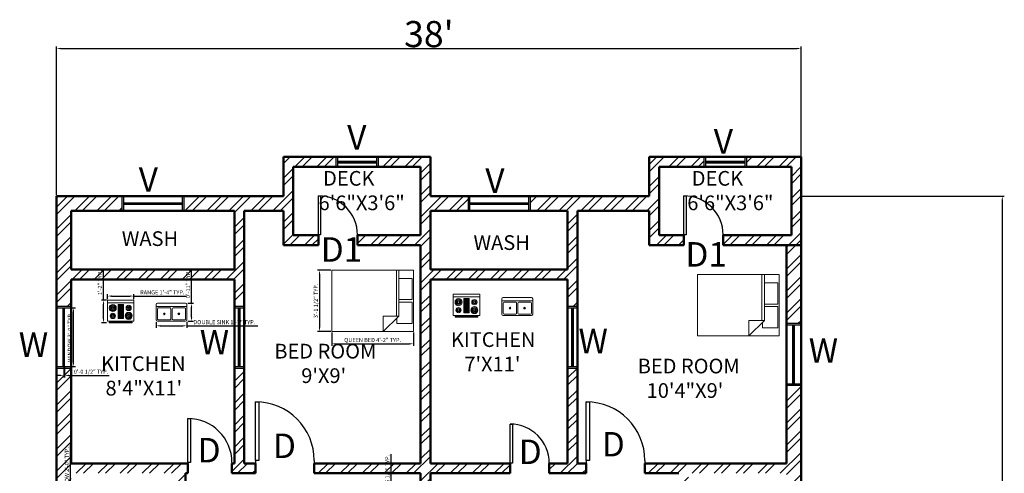
# Model space of a CAD drawing. Units: inches. Extents: x -31438 to -28352, y 12489 to 13610.
# Tile 3 of 5: x -31437 to -30834, y 13238 to 13516. Entities that reach past the tile are written whole.
import ezdxf

# ---------------------------------------------------------------- set-up
doc = ezdxf.new("R2010")
doc.units = ezdxf.units.IN
for name, color, linetype, lineweight in [('A-ANNO-DIMS', 2, 'Continuous', 18), ('A-ANNO-TEXT', 7, 'Continuous', 18), ('A-AREA-IDEN', 3, 'Continuous', 18), ('A-DOOR', 3, 'Continuous', 25), ('A-FLOR-FIXT', 9, 'Continuous', 18), ('A-FURN', 8, 'Continuous', 18), ('A-GLAZ', 4, 'Continuous', 25), ('A-WALL', 7, 'Continuous', 50), ('A-WALL-PATT', 8, 'Continuous', 13)]:
    doc.layers.add(name, color=color, linetype=linetype, lineweight=lineweight)
doc.styles.get("Standard").update_dxf_attribs({"font": 'arial.ttf'})
doc.dimstyles.new('ISO-25', dxfattribs={"dimtxt": 2.5, "dimasz": 2.5, "dimexe": 1.25, "dimexo": 0.625, "dimtad": 1, "dimdec": 0, "dimlunit": 3, "dimtxsty": 'Standard', "dimcen": 2.5, "dimadec": 0, "dimazin": 0, "dimtfac": 1, "dimtdec": 0, "dimtmove": 0, "dimatfit": 3, "dimfxl": 1, "dimarcsym": 0})

# ---------------------------------------------------------------- blocks, each defined once
blk = doc.blocks.new('*U8')
for p, q in [((0, 0), (0, -100)), ((750, 0), (750, -100))]:
    blk.add_line(p, q)
blk.add_lwpolyline([(0, 0), (0, 750), (43.75, 750), (43.75, 0)], close=True)
blk.add_arc((0, 0), 750, 0, 90)
blk = doc.blocks.new('Bed - Queen')
for p, q in [((0, -80.00003), (0, 0)), ((0, 0), (59.99999, 0)), ((59.99999, 0), (59.99999, -80.00003)), ((7.99999, -1.2), (28.79998, -1.2)), ((7.99999, -14.4), (7.99999, -1.2)), ((28.79998, -1.2), (28.79998, -14.4)), ((31.19999, -1.2), (51.99999, -1.2)), ((31.19999, -14.4), (31.19999, -1.2)), ((51.99999, -1.2), (51.99999, -16.4)), ((0, -14.4), (44.8, -14.4)), ((44.8, -16.8), (0, -16.8)), ((59.99999, -29.6), (44.8, -14.4)), ((44.8, -14.4), (44.8, -29.6)), ((51.99999, -16.4), (46.79936, -16.4)), ((44.8, -29.6), (59.99999, -29.6)), ((59.99999, -80.00003), (0, -80.00003))]:
    blk.add_line(p, q)
blk = doc.blocks.new('Range-Oven - 30 in top')
for p, q in [((0, -3), (30, -3)), ((12, -6), (18, -6)), ((13, -20), (13, -6)), ((14, -6), (14, -20)), ((15, -20), (15, -6)), ((16, -6), (16, -20)), ((17, -20), (17, -6)), ((18, -20), (12, -20)), ((6, -24), (6, -25)), ((8, -25), (8, -24)), ((22, -25), (22, -24)), ((24, -24), (24, -25))]:
    blk.add_line(p, q)
for points in [[(0, -24), (0, 0), (30, 0), (30, -24)], [(12, -21), (12, -5), (18, -5), (18, -21)], [(2, -26), (2, -25), (28, -25), (28, -26)]]:
    blk.add_lwpolyline(points, close=True)
for centre, radius in [((6, -9), 4), ((6, -9), 3), ((6, -9), 2), ((6, -9), 1), ((24, -9), 3), ((24, -9), 2), ((24, -9), 1), ((6, -18), 3), ((6, -18), 2), ((6, -18), 1), ((24, -18), 4), ((24, -18), 3), ((24, -18), 2), ((24, -18), 1)]:
    blk.add_circle(centre, radius)
blk = doc.blocks.new('Sink-double - 36 in top')
for p, q in [((-18, -4), (18, -4)), ((-0.75, -18.5), (-0.75, -6.5)), ((0.75, -6.5), (0.75, -18.5))]:
    blk.add_line(p, q)
for points in [[(-16.5, 0), (16.5, 0)], [(-18, -19.5), (-18, -1.5)], [(-16.5, -18.5), (-16.5, -6.5)], [(-15.5, -5.5), (-1.75, -5.5)], [(1.75, -5.5), (15.5, -5.5)], [(16.5, -6.5), (16.5, -18.5)], [(18, -1.5), (18, -19.5)], [(16.5, -21), (-16.5, -21)], [(-1.75, -19.5), (-15.5, -19.5)], [(15.5, -19.5), (1.75, -19.5)]]:
    blk.add_lwpolyline(points)
for centre, radius in [((-8.5, -12.5), 1), ((8.5, -12.5), 1), ((-8.5, -12.5), 0.5), ((8.5, -12.5), 0.5)]:
    blk.add_circle(centre, radius)
for centre, radius, start, end in [((-16.5, -1.5), 1.5, 90, 180), ((16.5, -1.5), 1.5, 0, 90), ((-15.5, -6.5), 1, 90, 180), ((-1.75, -6.5), 1, 0, 90), ((1.75, -6.5), 1, 90, 180), ((15.5, -6.5), 1, 0, 90), ((-16.5, -19.5), 1.5, 180, 270), ((-15.5, -18.5), 1, 180, 270), ((-1.75, -18.5), 1, 270, 0), ((1.75, -18.5), 1, 180, 270), ((15.5, -18.5), 1, 270, 0), ((16.5, -19.5), 1.5, 270, 0)]:
    blk.add_arc(centre, radius, start, end)
blk = doc.blocks.new('*D170')
at = {"layer": 'A-ANNO-DIMS', "color": 0, "lineweight": -2, "transparency": 16777216}
for p, q in [((-31414.86, 13408.54), (-31414.86, 13499.66)), ((-30958.86, 13408.54), (-30958.86, 13499.66)), ((-31412.36, 13498.41), (-30961.36, 13498.41))]:
    blk.add_line(p, q, dxfattribs=at)
at = {"layer": 'A-ANNO-DIMS', "color": 0, "transparency": 16777216}
for points in [[(-31412.36, 13498.83), (-31412.36, 13497.99), (-31414.86, 13498.41)], [(-30961.36, 13498.83), (-30961.36, 13497.99), (-30958.86, 13498.41)]]:
    blk.add_solid(points, dxfattribs=at)
at = {"layer": 'Defpoints', "color": 0, "transparency": 16777216}
for p in [(-30958.86, 13498.41), (-31414.86, 13407.92), (-30958.86, 13407.92)]:
    blk.add_point(p, dxfattribs=at)
at = {"layer": 'A-ANNO-DIMS', "color": 0, "transparency": 16777216, "insert": (-31186.86, 13507.21), "char_height": 2.5, "attachment_point": 5}
blk.add_mtext("{\\H6.4x;38'}", dxfattribs=at)
blk = doc.blocks.new('*D171')
at = {"layer": 'A-ANNO-DIMS', "color": 0, "lineweight": -2, "transparency": 16777216}
for p, q in [((-30958.23, 13407.92), (-30834.47, 13407.92)), ((-30835.72, 13405.42), (-30835.72, 12570.42)), ((-30958.23, 12567.92), (-30834.47, 12567.92))]:
    blk.add_line(p, q, dxfattribs=at)
at = {"layer": 'A-ANNO-DIMS', "color": 0, "transparency": 16777216}
for points in [[(-30836.13, 13405.42), (-30835.3, 13405.42), (-30835.72, 13407.92)], [(-30836.13, 12570.42), (-30835.3, 12570.42), (-30835.72, 12567.92)]]:
    blk.add_solid(points, dxfattribs=at)
at = {"layer": 'Defpoints', "color": 0, "transparency": 16777216}
for p in [(-30958.86, 13407.92), (-30958.86, 12567.92), (-30835.72, 12567.92)]:
    blk.add_point(p, dxfattribs=at)
at = {"layer": 'A-ANNO-DIMS', "color": 0, "transparency": 16777216, "insert": (-30844.51, 12987.92), "char_height": 2.5, "attachment_point": 5, "rotation": 90}
blk.add_mtext("{\\H6.4x;70'}", dxfattribs=at)
blk = doc.blocks.new('WIN-36')
for p, q in [((0, 0), (0, 36)), ((0.5, 0), (0.5, 36))]:
    blk.add_line(p, q)
blk = doc.blocks.new('*D182')
at = {"layer": 'A-ANNO-DIMS', "color": 0, "lineweight": -2, "transparency": 16777216}
for p, q in [((-31209.96, 13225.29), (-31209.96, 13249.87)), ((-31213.84, 13225.29), (-31208.71, 13225.29)), ((-31209.96, 13209.45), (-31209.96, 13222.79)), ((-31213.84, 13206.95), (-31208.71, 13206.95))]:
    blk.add_line(p, q, dxfattribs=at)
at = {"layer": 'A-ANNO-DIMS', "color": 0, "transparency": 16777216}
for points in [[(-31210.38, 13222.79), (-31209.55, 13222.79), (-31209.96, 13225.29)], [(-31210.38, 13209.45), (-31209.55, 13209.45), (-31209.96, 13206.95)]]:
    blk.add_solid(points, dxfattribs=at)
at = {"layer": 'Defpoints', "color": 0, "transparency": 16777216}
for p in [(-31214.46, 13225.29), (-31209.96, 13225.29), (-31214.46, 13206.95)]:
    blk.add_point(p, dxfattribs=at)
at = {"layer": 'A-ANNO-DIMS', "color": 0, "transparency": 16777216, "insert": (-31211.88, 13238.83), "char_height": 2.5, "attachment_point": 5, "rotation": 90}
blk.add_mtext('1\'-6 1/2" TYP.', dxfattribs=at)
blk = doc.blocks.new('*D185')
at = {"layer": 'A-ANNO-DIMS', "color": 0, "lineweight": -2, "transparency": 16777216}
for p, q in [((-31246.31, 13324.33), (-31246.31, 13316.19)), ((-31196.21, 13324.33), (-31196.21, 13316.19)), ((-31243.81, 13317.44), (-31198.71, 13317.44))]:
    blk.add_line(p, q, dxfattribs=at)
at = {"layer": 'A-ANNO-DIMS', "color": 0, "transparency": 16777216}
for points in [[(-31243.81, 13317.86), (-31243.81, 13317.02), (-31246.31, 13317.44)], [(-31198.71, 13317.86), (-31198.71, 13317.02), (-31196.21, 13317.44)]]:
    blk.add_solid(points, dxfattribs=at)
at = {"layer": 'Defpoints', "color": 0, "transparency": 16777216}
for p in [(-31246.31, 13324.96), (-31196.21, 13324.96), (-31196.21, 13317.44)]:
    blk.add_point(p, dxfattribs=at)
at = {"layer": 'A-ANNO-DIMS', "color": 0, "transparency": 16777216, "insert": (-31221.26, 13319.44), "char_height": 2.5, "attachment_point": 5}
blk.add_mtext('QUEEN BED 4\'-2" TYP.', dxfattribs=at)
blk = doc.blocks.new('*D186')
at = {"layer": 'A-ANNO-DIMS', "color": 0, "lineweight": -2, "transparency": 16777216}
for p, q in [((-31246.93, 13362.53), (-31255.07, 13362.53)), ((-31253.82, 13360.03), (-31253.82, 13327.46)), ((-31246.93, 13324.96), (-31255.07, 13324.96))]:
    blk.add_line(p, q, dxfattribs=at)
at = {"layer": 'A-ANNO-DIMS', "color": 0, "transparency": 16777216}
for points in [[(-31254.24, 13360.03), (-31253.41, 13360.03), (-31253.82, 13362.53)], [(-31254.24, 13327.46), (-31253.41, 13327.46), (-31253.82, 13324.96)]]:
    blk.add_solid(points, dxfattribs=at)
at = {"layer": 'Defpoints', "color": 0, "transparency": 16777216}
for p in [(-31246.31, 13362.53), (-31253.82, 13324.96), (-31246.31, 13324.96)]:
    blk.add_point(p, dxfattribs=at)
at = {"layer": 'A-ANNO-DIMS', "color": 0, "transparency": 16777216, "insert": (-31255.74, 13343.74), "char_height": 2.5, "attachment_point": 5, "rotation": 90}
blk.add_mtext('3\'-1 1/2" TYP.', dxfattribs=at)
blk = doc.blocks.new('*D193')
at = {"layer": 'A-ANNO-DIMS', "color": 0, "lineweight": -2, "transparency": 16777216}
for p, q in [((-31406.26, 13220.1), (-31406.26, 13255.48)), ((-31409.23, 13220.1), (-31405.01, 13220.1)), ((-31406.26, 13198.6), (-31406.26, 13217.6)), ((-31409.23, 13196.1), (-31405.01, 13196.1))]:
    blk.add_line(p, q, dxfattribs=at)
at = {"layer": 'A-ANNO-DIMS', "color": 0, "transparency": 16777216}
for points in [[(-31406.67, 13217.6), (-31405.84, 13217.6), (-31406.26, 13220.1)], [(-31406.67, 13198.6), (-31405.84, 13198.6), (-31406.26, 13196.1)]]:
    blk.add_solid(points, dxfattribs=at)
at = {"layer": 'Defpoints', "color": 0, "transparency": 16777216}
for p in [(-31409.86, 13220.1), (-31406.26, 13220.1), (-31409.86, 13196.1)]:
    blk.add_point(p, dxfattribs=at)
at = {"layer": 'A-ANNO-DIMS', "color": 0, "transparency": 16777216, "insert": (-31408.17, 13239.04), "char_height": 2.5, "attachment_point": 5, "rotation": 90}
blk.add_mtext('WINDOW 2\'-0" TYP.', dxfattribs=at)
blk = doc.blocks.new('*D195')
at = {"layer": 'A-ANNO-DIMS', "color": 0, "lineweight": -2, "transparency": 16777216}
for p, q in [((-31409.23, 13339.51), (-31403.21, 13339.51)), ((-31404.46, 13306.01), (-31404.46, 13337.01)), ((-31409.23, 13303.51), (-31403.21, 13303.51))]:
    blk.add_line(p, q, dxfattribs=at)
at = {"layer": 'A-ANNO-DIMS', "color": 0, "transparency": 16777216}
for points in [[(-31404.87, 13337.01), (-31404.04, 13337.01), (-31404.46, 13339.51)], [(-31404.87, 13306.01), (-31404.04, 13306.01), (-31404.46, 13303.51)]]:
    blk.add_solid(points, dxfattribs=at)
at = {"layer": 'Defpoints', "color": 0, "transparency": 16777216}
for p in [(-31409.86, 13339.51), (-31404.46, 13339.51), (-31409.86, 13303.51)]:
    blk.add_point(p, dxfattribs=at)
at = {"layer": 'A-ANNO-DIMS', "color": 0, "transparency": 16777216, "insert": (-31406.38, 13321.51), "char_height": 2.5, "attachment_point": 5, "rotation": 90}
blk.add_mtext('WINDOW 3\'-0" TYP.', dxfattribs=at)
blk = doc.blocks.new('*D196')
at = {"layer": 'A-ANNO-DIMS', "color": 0, "lineweight": -2, "transparency": 16777216}
for p, q in [((-31410.36, 13302.88), (-31410.36, 13296.86)), ((-31409.86, 13302.88), (-31409.86, 13296.86)), ((-31412.86, 13298.11), (-31415.36, 13298.11)), ((-31410.36, 13298.11), (-31409.86, 13298.11)), ((-31407.36, 13298.11), (-31382.54, 13298.11))]:
    blk.add_line(p, q, dxfattribs=at)
at = {"layer": 'A-ANNO-DIMS', "color": 0, "transparency": 16777216}
for points in [[(-31412.86, 13298.52), (-31412.86, 13297.69), (-31410.36, 13298.11)], [(-31407.36, 13298.52), (-31407.36, 13297.69), (-31409.86, 13298.11)]]:
    blk.add_solid(points, dxfattribs=at)
at = {"layer": 'Defpoints', "color": 0, "transparency": 16777216}
for p in [(-31410.36, 13303.51), (-31409.86, 13303.51), (-31409.86, 13298.11)]:
    blk.add_point(p, dxfattribs=at)
at = {"layer": 'A-ANNO-DIMS', "color": 0, "transparency": 16777216, "insert": (-31393.7, 13300.02), "char_height": 2.5, "attachment_point": 5}
blk.add_mtext('0\'-0 1/2" TYP.', dxfattribs=at)
blk = doc.blocks.new('*D197')
at = {"layer": 'A-ANNO-DIMS', "color": 0, "lineweight": -2, "transparency": 16777216}
for p, q in [((-31383.61, 13344.88), (-31383.61, 13347.94)), ((-31381.11, 13346.69), (-31369.92, 13346.69)), ((-31367.42, 13344.88), (-31367.42, 13347.94)), ((-31367.42, 13346.69), (-31335.17, 13346.69))]:
    blk.add_line(p, q, dxfattribs=at)
at = {"layer": 'A-ANNO-DIMS', "color": 0, "transparency": 16777216}
for points in [[(-31381.11, 13347.11), (-31381.11, 13346.27), (-31383.61, 13346.69)], [(-31369.92, 13347.11), (-31369.92, 13346.27), (-31367.42, 13346.69)]]:
    blk.add_solid(points, dxfattribs=at)
at = {"layer": 'Defpoints', "color": 0, "transparency": 16777216}
for p in [(-31383.61, 13344.26), (-31367.42, 13346.69), (-31367.42, 13344.26)]:
    blk.add_point(p, dxfattribs=at)
at = {"layer": 'A-ANNO-DIMS', "color": 0, "transparency": 16777216, "insert": (-31350.04, 13348.61), "char_height": 2.5, "attachment_point": 5}
blk.add_mtext('RANGE 1\'-4" TYP.', dxfattribs=at)
blk = doc.blocks.new('*D198')
at = {"layer": 'A-ANNO-DIMS', "color": 0, "lineweight": -2, "transparency": 16777216}
for p, q in [((-31386.04, 13344.26), (-31386.04, 13363.01)), ((-31384.24, 13344.26), (-31387.29, 13344.26)), ((-31386.04, 13332.72), (-31386.04, 13341.76)), ((-31384.24, 13330.22), (-31387.29, 13330.22))]:
    blk.add_line(p, q, dxfattribs=at)
at = {"layer": 'A-ANNO-DIMS', "color": 0, "transparency": 16777216}
for points in [[(-31386.46, 13341.76), (-31385.62, 13341.76), (-31386.04, 13344.26)], [(-31386.46, 13332.72), (-31385.62, 13332.72), (-31386.04, 13330.22)]]:
    blk.add_solid(points, dxfattribs=at)
at = {"layer": 'Defpoints', "color": 0, "transparency": 16777216}
for p in [(-31386.04, 13344.26), (-31383.61, 13344.26), (-31383.61, 13330.22)]:
    blk.add_point(p, dxfattribs=at)
at = {"layer": 'A-ANNO-DIMS', "color": 0, "transparency": 16777216, "insert": (-31387.92, 13354.89), "char_height": 2.5, "attachment_point": 5, "rotation": 90}
blk.add_mtext('1\'-2" TYP.', dxfattribs=at)
blk = doc.blocks.new('*D205')
at = {"layer": 'A-ANNO-DIMS', "color": 0, "lineweight": -2, "transparency": 16777216}
for p, q in [((-31353.83, 13330.68), (-31353.83, 13327.23)), ((-31334.97, 13330.68), (-31334.97, 13327.23)), ((-31351.33, 13328.48), (-31337.47, 13328.48)), ((-31334.97, 13328.48), (-31291.66, 13328.48))]:
    blk.add_line(p, q, dxfattribs=at)
at = {"layer": 'A-ANNO-DIMS', "color": 0, "transparency": 16777216}
for points in [[(-31351.33, 13328.89), (-31351.33, 13328.06), (-31353.83, 13328.48)], [(-31337.47, 13328.89), (-31337.47, 13328.06), (-31334.97, 13328.48)]]:
    blk.add_solid(points, dxfattribs=at)
at = {"layer": 'Defpoints', "color": 0, "transparency": 16777216}
for p in [(-31353.83, 13331.3), (-31334.97, 13331.3), (-31334.97, 13328.48)]:
    blk.add_point(p, dxfattribs=at)
at = {"layer": 'A-ANNO-DIMS', "color": 0, "transparency": 16777216, "insert": (-31312.07, 13330.39), "char_height": 2.5, "attachment_point": 5}
blk.add_mtext('DOUBLE SINK 1\'-7" TYP.', dxfattribs=at)
blk = doc.blocks.new('*D206')
at = {"layer": 'A-ANNO-DIMS', "color": 0, "lineweight": -2, "transparency": 16777216}
for p, q in [((-31332.15, 13342.3), (-31332.15, 13363.23)), ((-31334.35, 13342.3), (-31330.9, 13342.3)), ((-31332.15, 13333.8), (-31332.15, 13339.8)), ((-31334.35, 13331.3), (-31330.9, 13331.3))]:
    blk.add_line(p, q, dxfattribs=at)
at = {"layer": 'A-ANNO-DIMS', "color": 0, "transparency": 16777216}
for points in [[(-31332.56, 13339.8), (-31331.73, 13339.8), (-31332.15, 13342.3)], [(-31332.56, 13333.8), (-31331.73, 13333.8), (-31332.15, 13331.3)]]:
    blk.add_solid(points, dxfattribs=at)
at = {"layer": 'Defpoints', "color": 0, "transparency": 16777216}
for p in [(-31334.97, 13342.3), (-31332.15, 13342.3), (-31334.97, 13331.3)]:
    blk.add_point(p, dxfattribs=at)
at = {"layer": 'A-ANNO-DIMS', "color": 0, "transparency": 16777216, "insert": (-31334.05, 13354.02), "char_height": 2.5, "attachment_point": 5, "rotation": 90}
blk.add_mtext('0\'-11" TYP.', dxfattribs=at)

msp = doc.modelspace()

# ---------------------------------------------------------------- hatches: boundary and pattern name
at = {"layer": 'A-WALL-PATT'}
h = msp.add_hatch(dxfattribs=at)
h.set_pattern_fill('ANSI32', color=256)
h.paths.add_polyline_path([(-30958.86, 13431.92), (-30992.36, 13431.92), (-30992.36, 13425.92), (-30964.86, 13425.92), (-30964.86, 13383.92), (-31006.63, 13383.92), (-31006.63, 13380.92), (-31006.63, 13377.92), (-30958.86, 13377.92)])
h.paths.add_polyline_path([(-30958.86, 13377.92), (-30967.86, 13377.92), (-30967.86, 13330.01), (-30958.86, 13330.01)])
h.paths.add_polyline_path([(-31018.36, 13431.92), (-31051.86, 13431.92), (-31051.86, 13407.92), (-31124.86, 13407.92), (-31124.86, 13398.92), (-31101.86, 13398.92), (-31101.86, 13362.92), (-31185.86, 13362.92), (-31185.86, 13398.92), (-31162.86, 13398.92), (-31162.86, 13407.92), (-31185.86, 13407.92), (-31185.86, 13431.92), (-31217.86, 13431.92), (-31217.86, 13425.92), (-31191.86, 13425.92), (-31191.86, 13383.92), (-31230.51, 13383.92), (-31230.51, 13377.92), (-31191.86, 13377.92), (-31191.86, 13244.1), (-31256.99, 13244.1), (-31256.99, 13238.1), (-31191.86, 13238.1), (-31191.86, 13183.6), (-31185.86, 13183.6), (-31185.86, 13238.1), (-31137.12, 13238.1), (-31137.12, 13244.1), (-31185.86, 13244.1), (-31185.86, 13356.92), (-31101.86, 13356.92), (-31101.86, 13340.51), (-31095.86, 13340.51), (-31095.86, 13398.92), (-31051.86, 13398.92), (-31051.86, 13377.92), (-31030.63, 13377.92), (-31030.63, 13383.92), (-31045.86, 13383.92), (-31045.86, 13425.92), (-31018.36, 13425.92)])
h.paths.add_polyline_path([(-31269.86, 13425.92), (-31243.86, 13425.92), (-31243.86, 13431.92), (-31275.86, 13431.92), (-31275.86, 13407.92), (-31336.86, 13407.92), (-31336.86, 13398.92), (-31305.86, 13398.92), (-31305.86, 13362.92), (-31405.86, 13362.92), (-31405.86, 13398.92), (-31374.86, 13398.92), (-31374.86, 13407.92), (-31414.86, 13407.92), (-31414.86, 13340.51), (-31405.86, 13340.51), (-31405.86, 13356.92), (-31305.86, 13356.92), (-31305.86, 13340.51), (-31299.86, 13340.51), (-31299.86, 13398.92), (-31275.86, 13398.92), (-31275.86, 13377.92), (-31254.51, 13377.92), (-31254.51, 13383.92), (-31269.86, 13383.92)])
h.paths.add_polyline_path([(-31299.86, 13302.51), (-31305.86, 13302.51), (-31305.86, 13244.1), (-31307.44, 13244.1), (-31307.44, 13241.1), (-31307.44, 13238.1), (-31292.99, 13238.1), (-31292.99, 13244.1), (-31299.86, 13244.1)])
h.paths.add_polyline_path([(-31334.44, 13244.1), (-31405.86, 13244.1), (-31405.86, 13302.51), (-31414.86, 13302.51), (-31414.86, 13221.1), (-31405.86, 13221.1), (-31405.86, 13238.1), (-31341.86, 13238.1), (-31341.86, 13213.77), (-31335.86, 13213.77), (-31335.86, 13238.1), (-31334.44, 13238.1)])
h.paths.add_polyline_path([(-31090.53, 13244.1), (-31095.86, 13244.1), (-31095.86, 13302.51), (-31101.86, 13302.51), (-31101.86, 13244.1), (-31113.12, 13244.1), (-31113.12, 13241.1), (-31113.12, 13238.1), (-31090.53, 13238.1)], flags=17)
h.paths.add_polyline_path([(-30958.86, 13292.01), (-30967.86, 13292.01), (-30967.86, 13244.1), (-31033.86, 13244.1), (-31054.53, 13244.1), (-31054.53, 13241.1), (-31054.53, 13238.1), (-31033.86, 13238.1), (-31033.86, 13218.45), (-31027.86, 13218.45), (-31027.86, 13238.1), (-30967.86, 13238.1), (-30967.86, 13221.1), (-30958.86, 13221.1)])
h.paths.add_polyline_path([(-30958.86, 13195.1), (-30967.86, 13195.1), (-30967.86, 13178.1), (-31027.86, 13178.1), (-31027.86, 13194.45), (-31030.86, 13194.45), (-31033.86, 13194.45), (-31033.86, 13162.82), (-31027.86, 13162.82), (-31027.86, 13172.1), (-30967.86, 13172.1), (-30967.86, 13147.51), (-30958.86, 13147.51)])
h.paths.add_polyline_path([(-30958.86, 13121.51), (-30967.86, 13121.51), (-30967.86, 13096.92), (-31027.86, 13096.92), (-31027.86, 13128.82), (-31033.86, 13128.82), (-31033.86, 13096.92), (-31037.31, 13096.92), (-31037.31, 13090.92), (-30967.86, 13090.92), (-30967.86, 13067.92), (-30958.86, 13067.92)])
h.paths.add_polyline_path([(-30958.86, 13029.92), (-30967.86, 13029.92), (-30967.86, 13006.92), (-31025.37, 13006.92), (-31095.86, 13006.92), (-31095.86, 13000.92), (-31081.86, 13000.92), (-31081.86, 12943.92), (-31095.86, 12943.92), (-31095.86, 12937.92), (-31081.86, 12937.92), (-31081.86, 12894.3), (-31075.86, 12894.3), (-31075.86, 13000.92), (-31025.37, 13000.92), (-30967.86, 13000.92), (-30967.86, 12946.42), (-30958.86, 12946.42)])
h.paths.add_polyline_path([(-31121.86, 13006.92), (-31135.86, 13006.92), (-31135.86, 13090.92), (-31081.86, 13090.92), (-31081.86, 13068.53), (-31075.86, 13068.53), (-31075.86, 13090.92), (-31073.31, 13090.92), (-31073.31, 13096.92), (-31141.86, 13096.92), (-31141.86, 13091.1), (-31147.29, 13091.1), (-31147.29, 13085.1), (-31141.86, 13085.1), (-31141.86, 12949.88), (-31146.05, 12949.88), (-31146.05, 12943.88), (-31141.86, 12943.88), (-31141.86, 12853.92), (-31185.86, 12853.92), (-31185.86, 12943.88), (-31182.05, 12943.88), (-31182.05, 12949.88), (-31192.89, 12949.88), (-31192.89, 12943.88), (-31191.86, 12943.88), (-31191.86, 12853.92), (-31231.86, 12853.92), (-31231.86, 12943.88), (-31228.89, 12943.88), (-31228.89, 12949.88), (-31231.86, 12949.88), (-31231.86, 12979.92), (-31272.86, 12979.92), (-31272.86, 12973.92), (-31237.86, 12973.92), (-31237.86, 12853.92), (-31298, 12853.92), (-31298, 12847.92), (-31191.86, 12847.92), (-31191.86, 12806.42), (-31185.86, 12806.42), (-31185.86, 12847.92), (-31074.17, 12847.92), (-31074.17, 12853.92), (-31075.86, 12853.92), (-31075.86, 12870.3), (-31081.86, 12870.3), (-31081.86, 12853.92), (-31135.86, 12853.92), (-31135.86, 12937.92), (-31121.86, 12937.92), (-31121.86, 12943.92), (-31135.86, 12943.92), (-31135.86, 13000.92), (-31121.86, 13000.92)])
h.paths.add_polyline_path([(-30958.86, 12908.42), (-30967.86, 12908.42), (-30967.86, 12853.92), (-31038.17, 12853.92), (-31038.17, 12850.92), (-31038.17, 12847.92), (-31033.86, 12847.92), (-31033.86, 12837.06), (-31027.86, 12837.06), (-31027.86, 12847.92), (-30967.86, 12847.92), (-30967.86, 12833.42), (-30958.86, 12833.42)])
h.paths.add_polyline_path([(-30958.86, 12807.42), (-30967.86, 12807.42), (-30967.86, 12792.92), (-31027.86, 12792.92), (-31027.86, 12803.06), (-31033.86, 12803.06), (-31033.86, 12773.49), (-31027.86, 12773.49), (-31027.86, 12786.92), (-30967.86, 12786.92), (-30967.86, 12769.92), (-30958.86, 12769.92)])
h.paths.add_polyline_path([(-30958.86, 12743.92), (-30967.86, 12743.92), (-30967.86, 12726.92), (-31027.86, 12726.92), (-31027.86, 12749.49), (-31033.86, 12749.49), (-31033.86, 12726.92), (-31035.47, 12726.92), (-31035.47, 12720.92), (-30967.86, 12720.92), (-30967.86, 12667.92), (-30958.86, 12667.92)])
h.paths.add_polyline_path([(-30958.86, 12629.92), (-30967.86, 12629.92), (-30967.86, 12618.92), (-31071.86, 12618.92), (-31071.86, 12612.92), (-30967.86, 12612.92), (-30967.86, 12576.92), (-31000.86, 12576.92), (-31000.86, 12567.92), (-30958.86, 12567.92)])
h.paths.add_polyline_path([(-31038.86, 12576.92), (-31071.86, 12576.92), (-31071.86, 12629.92), (-31077.86, 12629.92), (-31077.86, 12576.92), (-31101.86, 12576.92), (-31101.86, 12597.92), (-31115.03, 12597.92), (-31115.03, 12591.92), (-31107.86, 12591.92), (-31107.86, 12549.92), (-31133.86, 12549.92), (-31133.86, 12543.92), (-31101.86, 12543.92), (-31101.86, 12567.92), (-31038.86, 12567.92)])
h.paths.add_polyline_path([(-31159.86, 12549.92), (-31185.86, 12549.92), (-31185.86, 12591.92), (-31139.03, 12591.92), (-31139.03, 12597.92), (-31185.86, 12597.92), (-31185.86, 12720.92), (-31126.49, 12720.92), (-31126.49, 12726.92), (-31185.86, 12726.92), (-31185.86, 12768.42), (-31191.86, 12768.42), (-31191.86, 12726.92), (-31226.35, 12726.92), (-31226.35, 12720.92), (-31191.86, 12720.92), (-31191.86, 12618.92), (-31275.86, 12618.92), (-31275.86, 12720.92), (-31262.35, 12720.92), (-31262.35, 12726.92), (-31298.57, 12726.92), (-31298.57, 12720.92), (-31281.86, 12720.92), (-31281.86, 12576.92), (-31321.86, 12576.92), (-31321.86, 12597.92), (-31340.38, 12597.92), (-31340.38, 12591.92), (-31327.86, 12591.92), (-31327.86, 12549.92), (-31355.36, 12549.92), (-31355.36, 12543.92), (-31321.86, 12543.92), (-31321.86, 12567.92), (-31252.86, 12567.92), (-31252.86, 12576.92), (-31275.86, 12576.92), (-31275.86, 12612.92), (-31191.86, 12612.92), (-31191.86, 12576.92), (-31214.86, 12576.92), (-31214.86, 12567.92), (-31191.86, 12567.92), (-31191.86, 12543.92), (-31159.86, 12543.92)])
h.paths.add_polyline_path([(-31071.86, 12720.92), (-31071.47, 12726.92), (-31090.49, 12726.92), (-31090.49, 12720.92), (-31077.86, 12720.92), (-31077.86, 12667.92), (-31071.86, 12667.92)])
h.paths.add_polyline_path([(-31381.36, 12549.92), (-31408.86, 12549.92), (-31408.86, 12591.92), (-31364.38, 12591.92), (-31364.38, 12597.92), (-31414.86, 12597.92), (-31414.86, 12543.92), (-31381.36, 12543.92)])
h.paths.add_polyline_path([(-31405.86, 12640.42), (-31414.86, 12640.42), (-31414.86, 12597.92), (-31405.86, 12597.92)])
h.paths.add_polyline_path([(-31405.86, 12720.92), (-31334.57, 12720.92), (-31334.57, 12726.92), (-31339.86, 12726.92), (-31339.86, 12750.16), (-31345.86, 12750.16), (-31345.86, 12726.92), (-31405.86, 12726.92), (-31405.86, 12743.92), (-31414.86, 12743.92), (-31414.86, 12678.42), (-31405.86, 12678.42)])
h.paths.add_polyline_path([(-31339.86, 12806.09), (-31345.86, 12806.09), (-31345.86, 12792.92), (-31405.86, 12792.92), (-31405.86, 12807.42), (-31414.86, 12807.42), (-31414.86, 12769.92), (-31405.86, 12769.92), (-31405.86, 12786.92), (-31345.86, 12786.92), (-31345.86, 12774.16), (-31339.86, 12774.16)])
h.paths.add_polyline_path([(-31334, 12853.92), (-31345.86, 12853.92), (-31345.86, 12973.92), (-31310.86, 12973.92), (-31310.86, 12979.92), (-31405.86, 12979.92), (-31405.86, 13013.51), (-31414.86, 13013.51), (-31414.86, 12971.92), (-31405.86, 12971.92), (-31405.86, 12970.92), (-31409.86, 12970.92), (-31409.86, 12946.92), (-31410.86, 12946.92), (-31410.86, 12970.92), (-31414.86, 12970.92), (-31414.86, 12883.92), (-31405.86, 12883.92), (-31405.86, 12882.92), (-31414.86, 12882.92), (-31414.86, 12833.42), (-31405.86, 12833.42), (-31405.86, 12847.92), (-31345.86, 12847.92), (-31345.86, 12840.09), (-31339.86, 12840.09), (-31339.86, 12847.92), (-31334, 12847.92)])
h.paths.add_polyline_path([(-31351.86, 12937.92), (-31359.89, 12937.92), (-31359.89, 12943.92), (-31351.86, 12943.92), (-31351.86, 12973.92), (-31405.86, 12973.92), (-31405.86, 12943.92), (-31383.89, 12943.92), (-31383.89, 12937.92), (-31405.86, 12937.92), (-31405.86, 12853.92), (-31351.86, 12853.92)], flags=16)
h.paths.add_polyline_path([(-31386.16, 12876.52), (-31390.61, 12876.52), (-31389.24, 12872.41, -0.501323), (-31392.64, 12859.49, -0.132891), (-31394.07, 12859.49, -0.501317), (-31397.46, 12872.41), (-31396.09, 12876.52), (-31398.15, 12876.52), (-31398.15, 12875.49), (-31400.2, 12875.49), (-31400.2, 12876.18), (-31400.22, 12876.52), (-31400.54, 12876.52), (-31400.54, 12882), (-31386.16, 12882)], flags=0)
h.paths.add_polyline_path([(-31387.36, 12877.2), (-31399.17, 12877.2, -0.414214), (-31399.86, 12877.72), (-31399.86, 12880.63, -0.414214), (-31399.35, 12881.31), (-31387.53, 12881.31, -0.414214), (-31386.85, 12880.8), (-31386.85, 12877.89, -0.414214)], flags=0)
h.paths.add_polyline_path([(-31392.23, 12860.41, -0.215004), (-31394.48, 12860.41, -0.48008), (-31396.09, 12872.41), (-31390.61, 12872.41, -0.48008)], flags=0)
h.paths.add_polyline_path([(-31359.87, 12913.86), (-31361.27, 12913.86), (-31361.27, 12937.86), (-31359.87, 12937.86)], flags=0)
h.paths.add_polyline_path([(-31230.55, 13091.1), (-31335.86, 13091.1), (-31335.86, 13129.57), (-31341.86, 13129.57), (-31341.86, 13091.1), (-31405.86, 13091.1), (-31405.86, 13118.6), (-31414.86, 13118.6), (-31414.86, 13051.51), (-31405.86, 13051.51), (-31405.86, 13085.1), (-31230.55, 13085.1)])
h.paths.add_polyline_path([(-31335.86, 13189.77), (-31341.86, 13189.77), (-31341.86, 13178.1), (-31405.86, 13178.1), (-31405.86, 13195.1), (-31414.86, 13195.1), (-31414.86, 13144.6), (-31405.86, 13144.6), (-31405.86, 13172.1), (-31341.86, 13172.1), (-31341.86, 13163.57), (-31335.86, 13163.57)])
h.paths.add_polyline_path([(-31387.11, 12934.37), (-31352.82, 12934.37), (-31352.82, 12965.28), (-31387.11, 12965.28)], flags=8)
h.paths.add_polyline_path([(-31406.38, 12887.22), (-31351.66, 12887.22), (-31351.66, 12920.8), (-31406.38, 12920.8)], flags=24)

# ---------------------------------------------------------------- linework, layer by layer
at = {"layer": 'A-GLAZ'}
for p, q in [((-31243.86, 13431.92), (-31243.86, 13425.92)), ((-31242.86, 13431.92), (-31242.86, 13425.92)), ((-31242.86, 13429.42), (-31218.86, 13429.42)), ((-31242.86, 13428.92), (-31218.86, 13428.92)), ((-31242.86, 13428.42), (-31218.86, 13428.42)), ((-31218.86, 13431.92), (-31218.86, 13425.92)), ((-31217.86, 13431.92), (-31217.86, 13425.92)), ((-31018.36, 13431.92), (-31018.36, 13425.92)), ((-31017.36, 13431.92), (-31017.36, 13425.92)), ((-31017.36, 13429.42), (-30993.36, 13429.42)), ((-31017.36, 13428.92), (-30993.36, 13428.92)), ((-31017.36, 13428.42), (-30993.36, 13428.42)), ((-30993.36, 13431.92), (-30993.36, 13425.92)), ((-30992.36, 13431.92), (-30992.36, 13425.92)), ((-31374.86, 13407.92), (-31374.86, 13398.92)), ((-31373.86, 13407.92), (-31373.86, 13398.92)), ((-31373.86, 13403.92), (-31337.86, 13403.92)), ((-31337.86, 13407.92), (-31337.86, 13398.92)), ((-31336.86, 13407.92), (-31336.86, 13398.92)), ((-31162.86, 13407.92), (-31162.86, 13398.92)), ((-31161.86, 13407.92), (-31161.86, 13398.92)), ((-31161.86, 13403.92), (-31125.86, 13403.92)), ((-31125.86, 13407.92), (-31125.86, 13398.92)), ((-31124.86, 13407.92), (-31124.86, 13398.92)), ((-31414.86, 13340.51), (-31405.86, 13340.51)), ((-31414.86, 13339.51), (-31405.86, 13339.51)), ((-31410.86, 13303.51), (-31410.86, 13339.51)), ((-31305.86, 13340.51), (-31299.86, 13340.51)), ((-31305.86, 13339.51), (-31299.86, 13339.51)), ((-31303.36, 13303.51), (-31303.36, 13339.51)), ((-31302.86, 13303.51), (-31302.86, 13339.51)), ((-31302.36, 13303.51), (-31302.36, 13339.51)), ((-31101.86, 13340.51), (-31095.86, 13340.51)), ((-31101.86, 13339.51), (-31095.86, 13339.51)), ((-31099.36, 13303.51), (-31099.36, 13339.51)), ((-31098.86, 13303.51), (-31098.86, 13339.51)), ((-31098.36, 13303.51), (-31098.36, 13339.51)), ((-30967.86, 13330.01), (-30958.86, 13330.01)), ((-30967.86, 13329.01), (-30958.86, 13329.01)), ((-30963.86, 13293.01), (-30963.86, 13329.01)), ((-31414.86, 13303.51), (-31405.86, 13303.51)), ((-31414.86, 13302.51), (-31405.86, 13302.51)), ((-31305.86, 13303.51), (-31299.86, 13303.51)), ((-31305.86, 13302.51), (-31299.86, 13302.51)), ((-31101.86, 13303.51), (-31095.86, 13303.51)), ((-31101.86, 13302.51), (-31095.86, 13302.51)), ((-30967.86, 13293.01), (-30958.86, 13293.01)), ((-30967.86, 13292.01), (-30958.86, 13292.01))]:
    msp.add_line(p, q, dxfattribs=at)
at = {"layer": 'A-WALL'}
for p, q in [((-31275.86, 13431.92), (-31185.86, 13431.92)), ((-31275.86, 13407.92), (-31275.86, 13431.92)), ((-31185.86, 13407.92), (-31185.86, 13431.92)), ((-31051.86, 13431.92), (-31051.86, 13407.92)), ((-31051.86, 13431.92), (-30958.86, 13431.92)), ((-30958.86, 13431.92), (-30958.86, 12567.92)), ((-31269.86, 13425.92), (-31191.86, 13425.92)), ((-31269.86, 13383.92), (-31269.86, 13425.92)), ((-31191.86, 13383.92), (-31191.86, 13425.92)), ((-31045.86, 13425.92), (-31045.86, 13383.92)), ((-31045.86, 13425.92), (-30964.86, 13425.92)), ((-30964.86, 13425.92), (-30964.86, 13383.92)), ((-31414.86, 13407.92), (-31275.86, 13407.92)), ((-31414.86, 12543.92), (-31414.86, 13407.92)), ((-31185.86, 13407.92), (-31051.86, 13407.92)), ((-31405.86, 13398.92), (-31305.86, 13398.92)), ((-31405.86, 13362.92), (-31405.86, 13398.92)), ((-31305.86, 13362.92), (-31305.86, 13398.92)), ((-31299.86, 13244.1), (-31299.86, 13398.92)), ((-31299.86, 13398.92), (-31275.86, 13398.92)), ((-31275.86, 13377.92), (-31275.86, 13398.92)), ((-31185.86, 13398.92), (-31101.86, 13398.92)), ((-31185.86, 13362.92), (-31185.86, 13398.92)), ((-31101.86, 13362.92), (-31101.86, 13398.92)), ((-31095.86, 13244.1), (-31095.86, 13398.92)), ((-31095.86, 13398.92), (-31051.86, 13398.92)), ((-31051.86, 13398.92), (-31051.86, 13377.92)), ((-31269.86, 13383.92), (-31254.51, 13383.92)), ((-31254.51, 13383.92), (-31254.51, 13377.92)), ((-31230.51, 13383.92), (-31230.51, 13377.92)), ((-31230.51, 13383.92), (-31191.86, 13383.92)), ((-31045.86, 13383.92), (-31030.63, 13383.92)), ((-31030.63, 13383.92), (-31030.63, 13377.92)), ((-31006.63, 13383.92), (-31006.63, 13377.92)), ((-31006.63, 13383.92), (-30964.86, 13383.92)), ((-31275.86, 13377.92), (-31254.51, 13377.92)), ((-31230.51, 13377.92), (-31191.86, 13377.92)), ((-31191.86, 13244.1), (-31191.86, 13377.92)), ((-31051.86, 13377.92), (-31030.63, 13377.92)), ((-31006.63, 13377.92), (-30958.86, 13377.92)), ((-30967.86, 13377.92), (-30967.86, 13244.1)), ((-31405.86, 13362.92), (-31305.86, 13362.92)), ((-31185.86, 13362.92), (-31101.86, 13362.92)), ((-31405.86, 13244.1), (-31405.86, 13356.92)), ((-31405.86, 13356.92), (-31305.86, 13356.92)), ((-31305.86, 13244.1), (-31305.86, 13356.92)), ((-31185.86, 13244.1), (-31185.86, 13356.92)), ((-31185.86, 13356.92), (-31101.86, 13356.92)), ((-31101.86, 13244.1), (-31101.86, 13356.92)), ((-31334.44, 13244.1), (-31405.86, 13244.1)), ((-31334.44, 13244.1), (-31334.44, 13238.1)), ((-31305.86, 13244.1), (-31307.44, 13244.1)), ((-31307.44, 13244.1), (-31307.44, 13238.1)), ((-31292.99, 13244.1), (-31299.86, 13244.1)), ((-31292.99, 13244.1), (-31292.99, 13238.1)), ((-31191.86, 13244.1), (-31256.99, 13244.1)), ((-31256.99, 13244.1), (-31256.99, 13238.1)), ((-31137.12, 13244.1), (-31185.86, 13244.1)), ((-31137.12, 13244.1), (-31137.12, 13238.1)), ((-31101.86, 13244.1), (-31113.12, 13244.1)), ((-31113.12, 13244.1), (-31113.12, 13238.1)), ((-31090.53, 13244.1), (-31095.86, 13244.1)), ((-31090.53, 13244.1), (-31090.53, 13238.1)), ((-31033.86, 13244.1), (-31054.53, 13244.1)), ((-31054.53, 13244.1), (-31054.53, 13238.1)), ((-30967.86, 13244.1), (-31033.86, 13244.1)), ((-31334.44, 13238.1), (-31335.86, 13238.1)), ((-31335.86, 13213.77), (-31335.86, 13238.1)), ((-31292.99, 13238.1), (-31307.44, 13238.1)), ((-31191.86, 13238.1), (-31256.99, 13238.1)), ((-31191.86, 13091.1), (-31191.86, 13238.1)), ((-31185.86, 13091.1), (-31185.86, 13238.1)), ((-31137.12, 13238.1), (-31185.86, 13238.1)), ((-31090.53, 13238.1), (-31113.12, 13238.1)), ((-31033.86, 13238.1), (-31054.53, 13238.1))]:
    msp.add_line(p, q, dxfattribs=at)

# ---------------------------------------------------------------- block references
at = {"layer": 'A-DOOR'}
for p, xscale, yscale, zscale in [((-31254.51, 13384.12), 0.0319999999999912, 0.0319999999999912, 0.0319999999999912), ((-31030.63, 13384.12), 0.0319999999999912, 0.0319999999999912, 0.0319999999999912), ((-31292.99, 13245.9), 0.0480000000000013, 0.0480000000000013, 0.0480000000000013), ((-31090.53, 13245.9), 0.0480000000000013, 0.0480000000000013, 0.0480000000000013), ((-31334.44, 13244.7), 0.036000000000001, 0.036000000000001, 0.036000000000001), ((-31137.12, 13244.3), 0.0319999999999686, 0.0319999999999686, 0.0319999999999686)]:
    msp.add_blockref('*U8', p, dxfattribs=dict(at, xscale=xscale, yscale=yscale, zscale=zscale))
at = {"layer": 'A-FLOR-FIXT'}
for name, p, xscale, yscale, zscale in [('Range-Oven - 30 in top', (-31383.61, 13344.26), 0.5398294676678127, 0.5398294676678127, 0.5398294676678127), ('Range-Oven - 30 in top', (-31171.9, 13347.81), 0.5398294676678127, 0.5398294676678127, 0.5398294676678127), ('Sink-double - 36 in top', (-31132.69, 13345.85), 0.5237879159203632, 0.5237879159203632, 0.5237879159203632), ('Sink-double - 36 in top', (-31344.4, 13342.3), 0.5237879159203632, 0.5237879159203632, 0.5237879159203632)]:
    msp.add_blockref(name, p, dxfattribs=dict(at, xscale=xscale, yscale=yscale, zscale=zscale))
at = {"layer": 'A-FURN', "xscale": 0.6262728017963775, "yscale": 0.6262728017963775, "zscale": 0.6262728017963775, "rotation": 270}
for p in [(-31196.21, 13362.53), (-30972.33, 13359.83)]:
    msp.add_blockref('Bed - Queen', p, dxfattribs=at)
at = {"layer": 'A-GLAZ', "rotation": 270}
for p in [(-31373.86, 13403.42), (-31161.86, 13403.42)]:
    msp.add_blockref('WIN-36', p, dxfattribs=at)
at = {"layer": 'A-GLAZ'}
for p in [(-31410.36, 13303.51), (-30963.36, 13293.01)]:
    msp.add_blockref('WIN-36', p, dxfattribs=at)

# ---------------------------------------------------------------- texts
at = {"layer": 'A-ANNO-TEXT', "char_height": 15, "attachment_point": 1}
for s, insert in [('{V}', (-31236.85, 13451.46)), ('{V}', (-31012.39, 13448.96)), ('{V}', (-31364.5, 13425.61)), ('{V}', (-31152.26, 13424.94)), ('{D1}', (-31253.04, 13382.74)), ('{D1}', (-31029.73, 13379.74)), ('{W}', (-31327.12, 13325.96)), ('{W}', (-31095.2, 13326.67)), ('{W}', (-31437.92, 13324.39)), ('{W}', (-30954.22, 13320.84)), ('{D}', (-31328.42, 13259.76)), ('{D}', (-31282.3, 13262.44)), ('{D}', (-31131.8, 13258.77)), ('{D}', (-31080.92, 13263.41))]:
    msp.add_mtext_dynamic_manual_height_columns(s, width=148.1867, gutter_width=12.5, heights=[0], dxfattribs=dict(at, insert=insert))
at = {"layer": 'A-AREA-IDEN', "char_height": 9, "attachment_point": 1}
for s, insert in [('{  DECK\\P 6\'6"X3\'6"}', (-31257.11, 13423.33)), ('{ DECK\\P6\'6"X3\'6"}', (-31028.6, 13423.33)), ('{WASH}', (-31374.87, 13386.39)), ('{WASH}', (-31159.5, 13383.96)), ("{KITCHEN\\P   7'X11'}", (-31173.33, 13324.53)), ("{BED ROOM\\P      9'X9'}", (-31281.47, 13317.44)), ('{KITCHEN\\P 8\'4"X11\'}', (-31387.58, 13309.78)), ('{BED ROOM\\P  10\'4"X9\'}', (-31058.98, 13308.33))]:
    msp.add_mtext_dynamic_manual_height_columns(s, width=1268.0892, gutter_width=12.5, heights=[0], dxfattribs=dict(at, insert=insert))

# ---------------------------------------------------------------- dimensions: what is measured, and where the dimension line sits
at = {"layer": 'A-ANNO-DIMS'}
for base, p1, p2, text, override, picture, middle in [((-30958.86, 13498.41), (-31414.86, 13407.92), (-30958.86, 13407.92), '{\\H6.4x;<>}', {"dimclrd": 0, "dimclre": 0, "dimclrt": 0}, '*D170', (-31186.86, 13507.21)), ((-31367.42, 13346.69), (-31383.61, 13344.26), (-31367.42, 13344.26), 'RANGE <> TYP.', {"dimdec": 1, "dimlfac": 1, "dimrnd": 0, "dimzin": 1, "dimdsep": 46, "dimlunit": 4, "dimfrac": 2}, '*D197', (-31350.04, 13348.61)), ((-31334.97, 13328.48), (-31353.83, 13331.3), (-31334.97, 13331.3), 'DOUBLE SINK <> TYP.', {"dimdec": 1, "dimlfac": 1, "dimrnd": 0, "dimzin": 1, "dimdsep": 46, "dimlunit": 4, "dimfrac": 2}, '*D205', (-31312.07, 13330.39)), ((-31196.21, 13317.44), (-31246.31, 13324.96), (-31196.21, 13324.96), 'QUEEN BED <> TYP.', {"dimdec": 1, "dimlfac": 1, "dimrnd": 0, "dimzin": 1, "dimdsep": 46, "dimlunit": 4, "dimfrac": 2}, '*D185', (-31221.26, 13319.44)), ((-31409.86, 13298.11), (-31410.36, 13303.51), (-31409.86, 13303.51), '<> TYP.', {"dimdec": 1, "dimlfac": 1, "dimrnd": 0, "dimzin": 1, "dimdsep": 46, "dimlunit": 4, "dimfrac": 2}, '*D196', (-31393.7, 13300.02))]:
    dim = msp.add_linear_dim(base=base, p1=p1, p2=p2, text=text, dimstyle='ISO-25', override=override, dxfattribs=at)
    dim.commit()
    dim.dimension.update_dxf_attribs({"geometry": picture, "text_midpoint": middle})
for base, p1, p2, angle, text, override, picture, middle in [((-30835.72, 12567.92), (-30958.86, 13407.92), (-30958.86, 12567.92), 90, '{\\H6.4x;<>}', {"dimclrd": 0, "dimclre": 0, "dimclrt": 0}, '*D171', (-30844.51, 12987.92)), ((-31386.04, 13344.26), (-31383.61, 13330.22), (-31383.61, 13344.26), 90, '<> TYP.', {"dimdec": 1, "dimlfac": 1, "dimrnd": 0, "dimzin": 1, "dimdsep": 46, "dimlunit": 4, "dimfrac": 2}, '*D198', (-31387.92, 13354.89)), ((-31332.15, 13342.3), (-31334.97, 13331.3), (-31334.97, 13342.3), 90, '<> TYP.', {"dimdec": 1, "dimlfac": 1, "dimrnd": 0, "dimzin": 1, "dimdsep": 46, "dimlunit": 4, "dimfrac": 2}, '*D206', (-31334.05, 13354.02)), ((-31253.82, 13324.96), (-31246.31, 13362.53), (-31246.31, 13324.96), 270, '<> TYP.', {"dimdec": 1, "dimlfac": 1, "dimrnd": 0, "dimzin": 1, "dimdsep": 46, "dimlunit": 4, "dimfrac": 2}, '*D186', (-31255.74, 13343.74)), ((-31404.46, 13339.51), (-31409.86, 13303.51), (-31409.86, 13339.51), 90, 'WINDOW <> TYP.', {"dimdec": 1, "dimlfac": 1, "dimrnd": 0, "dimzin": 1, "dimdsep": 46, "dimlunit": 4, "dimfrac": 2}, '*D195', (-31406.38, 13321.51)), ((-31406.26, 13220.1), (-31409.86, 13196.1), (-31409.86, 13220.1), 90, 'WINDOW <> TYP.', {"dimdec": 1, "dimlfac": 1, "dimrnd": 0, "dimzin": 1, "dimdsep": 46, "dimlunit": 4, "dimfrac": 2}, '*D193', (-31408.17, 13239.04)), ((-31209.96, 13225.29), (-31214.46, 13206.95), (-31214.46, 13225.29), 90, '<> TYP.', {"dimdec": 1, "dimlfac": 1, "dimrnd": 0, "dimzin": 1, "dimdsep": 46, "dimlunit": 4, "dimfrac": 2}, '*D182', (-31211.88, 13238.83))]:
    dim = msp.add_linear_dim(base=base, p1=p1, p2=p2, angle=angle, text=text, dimstyle='ISO-25', override=override, dxfattribs=at)
    dim.commit()
    dim.dimension.update_dxf_attribs({"geometry": picture, "text_midpoint": middle})

doc.saveas('drawing.dxf')
